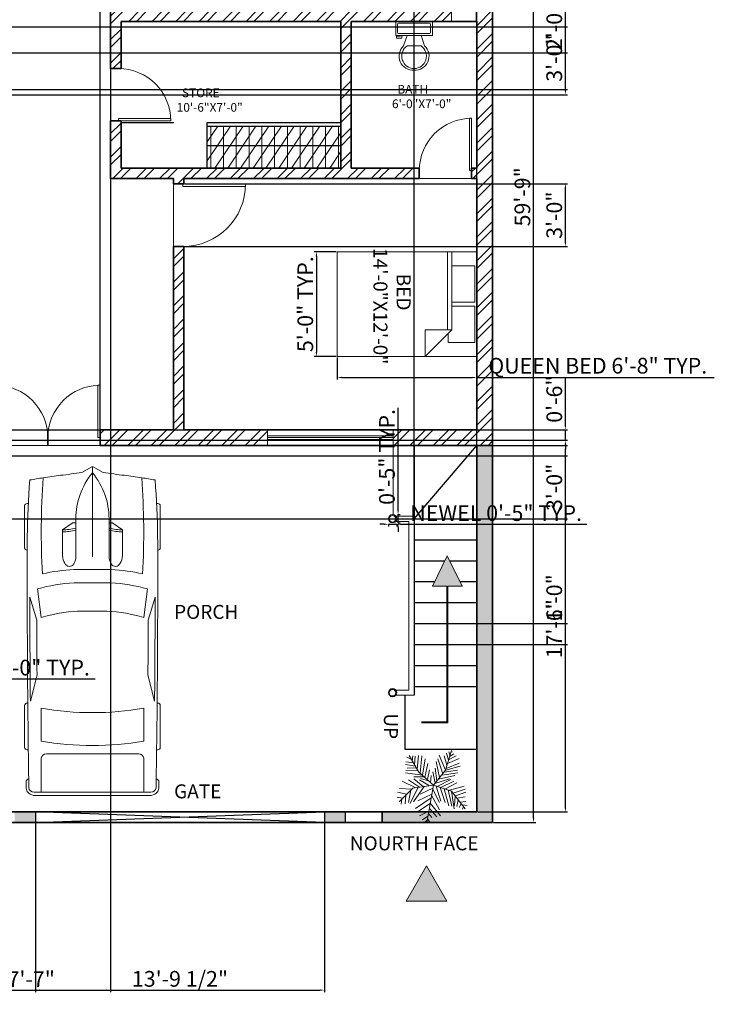
# Model space of a CAD drawing. Units: inches. Extents: x 177 to 1423, y 532 to 2503.
# Tile 3 of 5: x 453 to 852, y 532 to 1096. Entities that reach past the tile are written whole.
import ezdxf

# ---------------------------------------------------------------- set-up
doc = ezdxf.new("R2010")
doc.units = ezdxf.units.IN
for name, color, linetype, lineweight in [('A-ANNO-DIMS', 2, 'Continuous', 18), ('A-ANNO-SYMB', 7, 'Continuous', 18), ('A-ANNO-TEXT', 7, 'Continuous', 18), ('A-AREA-IDEN', 7, 'Continuous', 18), ('A-DOOR', 4, 'Continuous', 18), ('A-FLOR-CASE', 8, 'Continuous', 25), ('A-FLOR-CASE-PATT', 252, 'Continuous', 13), ('A-FLOR-FIXT', 9, 'Continuous', 18), ('A-FLOR-RAIL', 8, 'Continuous', 18), ('A-FLOR-STRS', 7, 'Continuous', 25), ('A-FURN', 8, 'Continuous', 18), ('A-GLAZ', 244, 'Continuous', 18), ('A-SITE-GATE', 244, 'Continuous', 25), ('A-WALL', 7, 'Continuous', 35), ('A-WALL-PATT', 252, 'Continuous', 13), ('C-SITE-VEHI', 9, 'Continuous', 13), ('L-PLNT', 94, 'Continuous', 13)]:
    doc.layers.add(name, color=color, linetype=linetype, lineweight=lineweight)
doc.styles.get("Standard").update_dxf_attribs({"font": 'arial.ttf'})
doc.dimstyles.new('ISO-25', dxfattribs={"dimtxt": 9, "dimasz": 2.5, "dimexe": 1.25, "dimexo": 0.625, "dimtad": 1, "dimlunit": 3, "dimtxsty": 'Standard', "dimcen": 2.5, "dimadec": 0, "dimazin": 0, "dimtfac": 1, "dimtmove": 0, "dimatfit": 3, "dimfxl": 1, "dimarcsym": 0})

# ---------------------------------------------------------------- blocks, each defined once
blk = doc.blocks.new('*U2')
for p, q in [((0, 0), (0, -6)), ((40, 0), (40, -6))]:
    blk.add_line(p, q)
blk.add_lwpolyline([(0, 0), (0, 40), (1.75, 40), (1.75, 0)], close=True)
blk.add_arc((0, 0), 40, 0, 90)
blk = doc.blocks.new('*U5')
for p, q in [((0, 0), (0, -6)), ((-40, 0), (-40, -6))]:
    blk.add_line(p, q)
blk.add_lwpolyline([(0, 0), (0, 40), (-1.75, 40), (-1.75, 0)], close=True)
blk.add_arc((0, 0), 40, 90, 180)
blk = doc.blocks.new('Bed - Queen')
for p, q in [((0, -80.00003), (0, 0)), ((0, 0), (59.99999, 0)), ((59.99999, 0), (59.99999, -80.00003)), ((7.99999, -1.2), (28.79998, -1.2)), ((7.99999, -14.4), (7.99999, -1.2)), ((28.79998, -1.2), (28.79998, -14.4)), ((31.19999, -1.2), (51.99999, -1.2)), ((31.19999, -14.4), (31.19999, -1.2)), ((51.99999, -1.2), (51.99999, -16.4)), ((0, -14.4), (44.8, -14.4)), ((44.8, -16.8), (0, -16.8)), ((59.99999, -29.6), (44.8, -14.4)), ((44.8, -14.4), (44.8, -29.6)), ((51.99999, -16.4), (46.79936, -16.4)), ((44.8, -29.6), (59.99999, -29.6)), ((59.99999, -80.00003), (0, -80.00003))]:
    blk.add_line(p, q)
blk = doc.blocks.new('*U9')
for p, q in [((9.5, -6), (9.5, -2)), ((-10, -8.5), (-8, -8.5)), ((-10, -9.5), (-10, -8.5)), ((-7, -9.5), (-10, -9.5)), ((-8, -8.5), (-8, -8)), ((-7, -8), (-7, -9.5)), ((-4, -8), (-6, -14)), ((4, -8), (6, -14)), ((4, -14), (-4, -14))]:
    blk.add_line(p, q)
blk.add_lwpolyline([(10.5, -8), (10.5, 0), (-10.5, 0), (-10.5, -8)], close=True)
for points in [[(-9.5, -2), (-9.5, -6)], [(8.5, -1), (-8.5, -1)], [(-8.5, -7), (8.5, -7)]]:
    blk.add_lwpolyline(points)
for centre, radius, start, end in [((-8.625, -1.875), 0.8839, 81.8699, 188.1301), ((8.625, -1.875), 0.8839, 351.8699, 98.1301), ((-8.625, -6.125), 0.8839, 171.869898, 278.1301), ((8.625, -6.125), 0.8839, 261.8699, 8.1301), ((-0.4772, -19.9188), 8.0953, 133.01722, 273.38), ((0.0374, -19.8731), 7.127, 124.50543, 269.7), ((-0.0373, -19.8731), 7.127, 270.3, 55.4946), ((0.4773, -19.9188), 8.0953, 266.62, 46.9828)]:
    blk.add_arc(centre, radius, start, end)
blk = doc.blocks.new('*U14')
for p, q in [((21.1, 37.41), (21.1, 36.83)), ((46.55, 38.89), (22.35, 38.89)), ((47.8, 37.39), (47.8, 37.41)), ((87.99, 31.87), (74.76, 35.92)), ((134.31, 35.6), (119.29, 31.78)), ((135.45, 37.07), (135.45, 37.41)), ((136.7, 38.89), (160.9, 38.89)), ((162.15, 37.41), (162.15, 36.77)), ((70.03, 31.54), (86.41, 29.35)), ((138.42, 29.35), (157.25, 29.35)), ((186.47, 29.35), (167.01, 29.35)), ((186.47, -33.5), (186.47, 33.5)), ((188.4, -32.76), (188.4, 32.76)), ((164.52, 26.39), (164.52, -26.39)), ((32.27, 11.63), (36.13, 17.17)), ((36.13, 17.17), (50.94, 17.17)), ((3.27, 6.13), (0.1, 0.41)), ((29.77, 9.51), (51.68, 9.51)), ((32.12, 9.51), (32.12, 11.15)), ((58.92, -10.77), (58.92, 10.77)), ((66.55, -10.53), (66.55, 10.53)), ((82.74, 8.5), (82.74, -8.5)), ((186.47, -10.53), (186.47, 10.53)), ((0, 0), (51.68, 0)), ((0.1, -0.41), (3.27, -6.13)), ((29.77, -9.51), (51.68, -9.51)), ((32.12, -9.51), (32.12, -11.15)), ((32.27, -11.63), (36.13, -17.17)), ((36.13, -17.17), (50.94, -17.17)), ((86.41, -29.35), (70.03, -31.54)), ((87.99, -31.87), (74.76, -35.92)), ((134.31, -35.6), (119.29, -31.78)), ((157.25, -29.35), (138.42, -29.35)), ((167.01, -29.35), (186.47, -29.35)), ((21.1, -37.41), (21.1, -36.83)), ((46.55, -38.89), (22.35, -38.89)), ((47.8, -37.39), (47.8, -37.41)), ((135.45, -37.07), (135.45, -37.41)), ((136.7, -38.89), (160.9, -38.89)), ((162.15, -37.41), (162.15, -36.77))]:
    blk.add_line(p, q)
for centre, major_axis, ratio, start_param, end_param in [((266.03, -27.52), (0, 313.31), 0.842304, 1.367076, 1.39176), ((41.19, -490.86), (0, 528.23), 0.842304, 0.00281, 0.075598), ((22.35, 37.41), (0, -1.48), 0.842304, 3.141593, 4.712389), ((64.48, -10555.62), (0, 10593.03), 0.842304, -0.013397, 0.002797), ((46.55, 37.41), (0, 1.48), 0.842304, -1.570796, 0), ((64.48, -10555.62), (0, -10591.55), 0.842304, 3.133765, 3.140441), ((136.7, 37.41), (0, -1.48), 0.842304, 3.141593, 4.712389), ((160.9, 37.41), (0, 1.48), 0.842304, -1.570796, 0), ((180.63, 35.84), (0, 2.22), 0.842304, -0.013017, 1.249894), ((64.48, -10556.36), (0, 10595.31), 0.842304, -0.013397, -0.013017), ((183.98, 33.5), (0, -2.96), 0.842304, 1.570796, 3.128196), ((183.98, 32.76), (0, -5.25), 0.842304, 1.570796, 3.128196), ((259.18, -27.52), (0, -305.3), 0.842304, 4.528606, 4.561838), ((37.47, -593.96), (0, -623.33), 0.842304, 3.096046, 3.200911), ((134.4, 5.39), (0, -89.78), 0.842304, 4.449482, 4.652344), ((135.29, 5.39), (0, 81.77), 0.842304, 1.245306, 1.50788), ((149.6, 2.8), (0, -79.58), 0.842304, 4.372215, 4.640744), ((95.79, -3666.35), (0, -3698.24), 0.842304, 3.134049, 3.144098), ((17.08, 0), (0, 147.02), 0.842304, 4.511394, 4.913384), ((35.91, 0), (0, 147.02), 0.842304, 4.511394, 4.913384), ((167.01, 26.39), (0, 2.96), 0.842304, 0, 1.570796), ((-204.49, 52.4), (0, -250.96), 0.842304, 1.385369, 1.434372), ((13.04, 17.01), (0, 27.42), 0.842304, 4.435146, 4.718221), ((14.2, 17.01), (0, 27.42), 0.842304, 4.435146, 4.718221), ((50.79, 13.34), (6.34, -0.36), 0.603834, -1.395552, 1.581315), ((32.75, 11.15), (0, 0.74), 0.842304, 0.879714, 1.570796), ((29.77, -46.66), (0, 56.17), 0.842304, 0, 0.590319), ((0.62, 0), (0, -0.74), 0.842304, 4.131459, 5.293319), ((29.77, 46.66), (0, 56.17), 0.842304, 2.551274, 3.141593), ((-204.49, -52.4), (0, 250.96), 0.842304, -1.434372, -1.385369), ((32.75, -11.15), (0, -0.74), 0.842304, 4.712389, 5.403472), ((13.04, -17.01), (0, -27.42), 0.842304, 1.564964, 1.848039), ((14.2, -17.01), (0, -27.42), 0.842304, 1.564964, 1.848039), ((134.4, -5.39), (0, -89.78), 0.842304, -1.510751, -1.307889), ((135.29, -5.39), (0, -81.77), 0.842304, -1.50788, -1.245306), ((149.6, -2.8), (0, -79.58), 0.842304, -1.499151, -1.230623), ((259.18, 27.52), (0, 305.3), 0.842304, 1.721348, 1.754579), ((167.01, -26.39), (0, -2.96), 0.842304, 4.712389, 6.283185), ((266.03, 27.52), (0, 313.31), 0.842304, 1.749832, 1.774517), ((37.47, 593.96), (0, -623.33), 0.842304, -0.059319, 0.045547), ((95.79, 3666.35), (0, -3698.24), 0.842304, -0.002505, 0.007544), ((183.98, -33.5), (0, 2.96), 0.842304, 3.15499, 4.712389), ((183.98, -32.76), (0, -5.25), 0.842304, 0.013397, 1.570796), ((41.19, 490.86), (0, -528.23), 0.842304, -0.075598, -0.00281), ((22.35, -37.41), (0, 1.48), 0.842304, 1.570796, 3.141593), ((64.48, 10555.62), (0, 10593.03), 0.842304, 3.138796, 3.15499), ((46.55, -37.41), (0, -1.48), 0.842304, 0, 1.570796), ((64.48, 10555.62), (0, -10591.55), 0.842304, 0.001152, 0.007828), ((136.7, -37.41), (0, -1.48), 0.842304, -1.570796, 0), ((160.9, -37.41), (0, 1.48), 0.842304, 3.141593, 4.712389), ((180.63, -35.84), (0, -2.22), 0.842304, -1.249894, 0.013017), ((64.48, 10556.36), (0, 10595.31), 0.842304, 3.15461, 3.15499)]:
    blk.add_ellipse(centre, major_axis=major_axis, ratio=ratio, start_param=start_param, end_param=end_param)
at = {"extrusion": (0, 0, -1)}
blk.add_ellipse((50.79, -13.34), major_axis=(6.34, 0.36), ratio=0.603834, start_param=-1.395552, end_param=1.581315, dxfattribs=at)
blk = doc.blocks.new('*D16')
at = {"layer": 'A-ANNO-DIMS', "color": 0, "lineweight": -2, "transparency": 16777216}
for p, q in [((725.18, 1353.15), (749.29, 1353.15)), ((748.04, 638.65), (748.04, 1350.65)), ((725.18, 636.15), (749.29, 636.15))]:
    blk.add_line(p, q, dxfattribs=at)
at = {"layer": 'A-ANNO-DIMS', "color": 0, "transparency": 16777216}
for points in [[(747.63, 1350.65), (748.46, 1350.65), (748.04, 1353.15)], [(747.63, 638.65), (748.46, 638.65), (748.04, 636.15)]]:
    blk.add_solid(points, dxfattribs=at)
at = {"layer": 'Defpoints', "color": 0, "transparency": 16777216}
for p in [(724.55, 1353.15), (748.04, 1353.15), (724.55, 636.15)]:
    blk.add_point(p, dxfattribs=at)
at = {"layer": 'A-ANNO-DIMS', "color": 0, "transparency": 16777216, "insert": (742.82, 994.65), "char_height": 9, "attachment_point": 5, "rotation": 90}
blk.add_mtext('59\'-9"', dxfattribs=at)
blk = doc.blocks.new('*U11')
for p, q in [((-7.288, 39.707), (-21.778, 46.673)), ((-8.737, 47.138), (-17.069, 52.711)), ((-10.186, 53.64), (-13.084, 55.962)), ((0, 0), (-10.5, 57)), ((-9.099, 51.782), (-6.563, 55.962)), ((-7.65, 43.423), (-2.578, 49.46)), ((-5.839, 35.992), (4.667, 48.067)), ((-5.114, 27.632), (10.463, 46.673)), ((-3.665, 19.273), (-27.574, 35.527)), ((-5.114, 28.097), (-24.676, 40.636)), ((-2.941, 16.486), (8.652, 37.85)), ((16.259, 5.805), (23.142, 31.348)), ((22.055, 7.198), (27.489, 32.277)), ((27, 9), (48, 36)), ((27.127, 9.056), (31.112, 35.992)), ((31.836, 30.883), (32.561, 16.486)), ((35.096, 32.741), (37.27, 22.524)), ((38.719, 34.134), (41.979, 28.561)), ((43.791, 29.954), (51.036, 30.883)), ((44.153, 36.456), (45.239, 32.741)), ((-47.498, 19.737), (-55.83, 18.344)), ((-31.5, 4.5), (-52.5, 25.5)), ((-48.585, 21.131), (-49.309, 29.026)), ((-43.513, 28.561), (-42.427, 15.558)), ((-38.442, 26.239), (-34.819, 7.663)), ((-35.544, 28.097), (-24.314, 3.947)), ((-14.533, 2.09), (-30.834, 25.31)), ((-24.314, 23.917), (-2.941, 13.7)), ((-1.129, 6.734), (9.014, 26.704)), ((3.942, 1.625), (11.187, 24.381)), ((10.101, 3.483), (17.708, 26.239)), ((33.285, 16.486), (48.862, 10.913)), ((36.183, 19.737), (48.137, 17.88)), ((40.53, 25.775), (48.862, 24.846)), ((-40.615, 13.7), (-55.105, 10.913)), ((-33.37, 6.269), (-52.207, 5.34)), ((-28.299, 3.483), (-47.86, -5.805)), ((-21.416, 3.018), (-38.079, -8.128)), ((0, 0), (-31.5, 4.5)), ((-15.982, 2.09), (-30.11, -9.521)), ((0, 0), (-22.5, -19.5)), ((-6.563, 1.161), (-21.416, -8.128)), ((-20.691, 13.7), (-1.129, 4.876)), ((0, 0), (27, 9)), ((0, 0), (18, -22.5)), ((6.478, 1.625), (26.04, -8.592)), ((11.187, 3.483), (30.749, -5.805)), ((18.07, 5.805), (35.096, -3.483)), ((24.229, 7.663), (46.688, 1.625)), ((29.662, 12.307), (48.137, 6.269)), ((-15.257, -12.772), (-30.11, -12.772)), ((-6.563, -5.805), (-19.967, -9.985)), ((-13.446, -11.378), (-8.737, -32.741)), ((-9.461, -8.592), (-6.201, -23.453)), ((-4.752, -3.483), (-3.665, -14.629)), ((2.493, -3.019), (-1.491, -20.202)), ((1.769, -2.555), (24.229, -9.521)), ((5.029, -6.27), (2.131, -25.775)), ((9.014, -11.378), (3.58, -35.992)), ((7.565, -9.056), (32.198, -14.629)), ((-17.431, -15.094), (-42.789, -18.809)), ((-28.299, -29.026), (-42.789, -31.348)), ((-24.314, -21.596), (-42.427, -22.06)), ((-26.849, -26.24), (-40.253, -25.775)), ((-22.5, -19.5), (-37.5, -45)), ((-25.038, -23.918), (-22.865, -45.281)), ((-20.691, -18.345), (-17.793, -44.352)), ((-17.069, -15.094), (-12.721, -40.172)), ((14.085, -16.951), (6.478, -40.172)), ((18.07, -22.524), (8.289, -45.745)), ((12.274, -15.094), (36.907, -18.809)), ((16.259, -19.738), (36.183, -22.989)), ((18, -22.5), (27, -52.5)), ((18.433, -22.524), (40.53, -29.026)), ((19.157, -25.311), (38.719, -33.206)), ((-30.834, -34.135), (-42.427, -35.528)), ((-34.457, -39.708), (-40.978, -42.494)), ((-32.646, -36.921), (-31.921, -44.352)), ((-29.023, -30.884), (-27.936, -43.887)), ((20.244, -30.419), (15.897, -44.816)), ((22.78, -37.85), (19.519, -48.532)), ((21.331, -32.741), (39.081, -40.636)), ((22.78, -38.314), (34.372, -44.816)), ((24.591, -43.423), (30.749, -47.603)), ((24.591, -45.745), (23.142, -50.854)), ((26.764, -49.925), (28.213, -50.854))]:
    blk.add_line(p, q)
blk = doc.blocks.new('WIN-GLAZING-72IN')
for p, q in [((72, 2), (0, 2)), ((72, 1), (0, 1)), ((72, 0), (0, 0))]:
    blk.add_line(p, q)
blk = doc.blocks.new('STAIR-NEWEL-ROUND')
for radius in [2.39, 1.89]:
    blk.add_circle((2.39, 2.39), radius)
blk = doc.blocks.new('*D22')
at = {"layer": 'A-ANNO-DIMS', "color": 0, "lineweight": -2, "transparency": 16777216}
for p, q in [((635.55, 902.53), (635.55, 889.9)), ((715.55, 902.53), (715.55, 889.9)), ((638.05, 891.15), (713.05, 891.15)), ((715.55, 891.15), (851.69, 891.15))]:
    blk.add_line(p, q, dxfattribs=at)
at = {"layer": 'A-ANNO-DIMS', "color": 0, "transparency": 16777216}
for points in [[(638.05, 891.57), (638.05, 890.74), (635.55, 891.15)], [(713.05, 891.57), (713.05, 890.74), (715.55, 891.15)]]:
    blk.add_solid(points, dxfattribs=at)
at = {"layer": 'Defpoints', "color": 0, "transparency": 16777216}
for p in [(635.55, 903.15), (715.55, 903.15), (715.55, 891.15)]:
    blk.add_point(p, dxfattribs=at)
at = {"layer": 'A-ANNO-DIMS', "color": 0, "transparency": 16777216, "insert": (784.87, 896.71), "char_height": 9, "attachment_point": 5}
blk.add_mtext('QUEEN BED 6\'-8" TYP.', dxfattribs=at)
blk = doc.blocks.new('*D23')
at = {"layer": 'A-ANNO-DIMS', "color": 0, "lineweight": -2, "transparency": 16777216}
for p, q in [((634.93, 963.15), (622.3, 963.15)), ((623.55, 960.65), (623.55, 905.65)), ((634.93, 903.15), (622.3, 903.15))]:
    blk.add_line(p, q, dxfattribs=at)
at = {"layer": 'A-ANNO-DIMS', "color": 0, "transparency": 16777216}
for points in [[(623.13, 960.65), (623.97, 960.65), (623.55, 963.15)], [(623.13, 905.65), (623.97, 905.65), (623.55, 903.15)]]:
    blk.add_solid(points, dxfattribs=at)
at = {"layer": 'Defpoints', "color": 0, "transparency": 16777216}
for p in [(635.55, 963.15), (623.55, 903.15), (635.55, 903.15)]:
    blk.add_point(p, dxfattribs=at)
at = {"layer": 'A-ANNO-DIMS', "color": 0, "transparency": 16777216, "insert": (618.33, 933.15), "char_height": 9, "attachment_point": 5, "rotation": 90}
blk.add_mtext('5\'-0" TYP.', dxfattribs=at)
blk = doc.blocks.new('*D24')
at = {"layer": 'A-ANNO-DIMS', "color": 0, "lineweight": -2, "transparency": 16777216}
for p, q in [((307.55, 708.28), (307.55, 719.7)), ((310.05, 718.45), (377.05, 718.45)), ((379.55, 708.28), (379.55, 719.7)), ((379.55, 718.45), (496.7, 718.45))]:
    blk.add_line(p, q, dxfattribs=at)
at = {"layer": 'A-ANNO-DIMS', "color": 0, "transparency": 16777216}
for points in [[(310.05, 718.87), (310.05, 718.04), (307.55, 718.45)], [(377.05, 718.87), (377.05, 718.04), (379.55, 718.45)]]:
    blk.add_solid(points, dxfattribs=at)
at = {"layer": 'Defpoints', "color": 0, "transparency": 16777216}
for p in [(379.55, 718.45), (307.55, 707.65), (379.55, 707.65)]:
    blk.add_point(p, dxfattribs=at)
at = {"layer": 'A-ANNO-DIMS', "color": 0, "transparency": 16777216, "insert": (439.37, 723.73), "char_height": 9, "attachment_point": 5}
blk.add_mtext('GLAZING 6\'-0" TYP.', dxfattribs=at)
blk = doc.blocks.new('*D28')
at = {"layer": 'A-ANNO-DIMS', "color": 0, "lineweight": -2, "transparency": 16777216}
for p, q in [((662.36, 807.04), (659.86, 807.04)), ((664.86, 807.13), (664.86, 805.79)), ((664.86, 807.04), (669.65, 807.04)), ((669.65, 807.13), (669.65, 805.79)), ((672.15, 807.04), (778.53, 807.04))]:
    blk.add_line(p, q, dxfattribs=at)
at = {"layer": 'A-ANNO-DIMS', "color": 0, "transparency": 16777216}
for points in [[(662.36, 807.46), (662.36, 806.62), (664.86, 807.04)], [(672.15, 807.46), (672.15, 806.62), (669.65, 807.04)]]:
    blk.add_solid(points, dxfattribs=at)
at = {"layer": 'Defpoints', "color": 0, "transparency": 16777216}
for p in [(664.86, 807.76), (669.65, 807.76), (669.65, 807.04)]:
    blk.add_point(p, dxfattribs=at)
at = {"layer": 'A-ANNO-DIMS', "color": 0, "transparency": 16777216, "insert": (726.59, 812.26), "char_height": 9, "attachment_point": 5}
blk.add_mtext('NEWEL 0\'-5" TYP.', dxfattribs=at)
blk = doc.blocks.new('*D29')
at = {"layer": 'A-ANNO-DIMS', "color": 0, "lineweight": -2, "transparency": 16777216}
for p, q in [((670.37, 815.05), (670.37, 873.66)), ((670.28, 812.55), (671.62, 812.55)), ((670.37, 807.76), (670.37, 812.55)), ((670.28, 807.76), (671.62, 807.76)), ((670.37, 805.26), (670.37, 802.76))]:
    blk.add_line(p, q, dxfattribs=at)
at = {"layer": 'A-ANNO-DIMS', "color": 0, "transparency": 16777216}
for points in [[(669.95, 815.05), (670.79, 815.05), (670.37, 812.55)], [(669.95, 805.26), (670.79, 805.26), (670.37, 807.76)]]:
    blk.add_solid(points, dxfattribs=at)
at = {"layer": 'Defpoints', "color": 0, "transparency": 16777216}
for p in [(669.65, 812.55), (670.37, 812.55), (669.65, 807.76)]:
    blk.add_point(p, dxfattribs=at)
at = {"layer": 'A-ANNO-DIMS', "color": 0, "transparency": 16777216, "insert": (665.15, 845.6), "char_height": 9, "attachment_point": 5, "rotation": 90}
blk.add_mtext('0\'-5" TYP.', dxfattribs=at)
blk = doc.blocks.new('*D35')
at = {"layer": 'A-ANNO-DIMS', "color": 0, "lineweight": -2, "transparency": 16777216}
for p, q in [((462.59, 635.53), (462.59, 538.84)), ((628.1, 635.53), (628.1, 538.84)), ((465.09, 540.09), (625.6, 540.09))]:
    blk.add_line(p, q, dxfattribs=at)
at = {"layer": 'A-ANNO-DIMS', "color": 0, "transparency": 16777216}
for points in [[(465.09, 540.51), (465.09, 539.68), (462.59, 540.09)], [(625.6, 540.51), (625.6, 539.68), (628.1, 540.09)]]:
    blk.add_solid(points, dxfattribs=at)
at = {"layer": 'Defpoints', "color": 0, "transparency": 16777216}
for p in [(462.59, 636.15), (628.1, 636.15), (628.1, 540.09)]:
    blk.add_point(p, dxfattribs=at)
at = {"layer": 'A-ANNO-DIMS', "color": 0, "transparency": 16777216, "insert": (545.34, 545.37), "char_height": 9, "attachment_point": 5}
blk.add_mtext('13\'-9 1/2"', dxfattribs=at)
blk = doc.blocks.new('*D36')
at = {"layer": 'A-ANNO-DIMS', "color": 0, "lineweight": -2, "transparency": 16777216}
for p, q in [((766.3, 750.15), (766.3, 776.98)), ((716.18, 750.15), (767.55, 750.15)), ((766.3, 740.65), (766.3, 747.65)), ((716.18, 738.15), (767.55, 738.15))]:
    blk.add_line(p, q, dxfattribs=at)
at = {"layer": 'A-ANNO-DIMS', "color": 0, "transparency": 16777216}
for points in [[(765.88, 747.65), (766.72, 747.65), (766.3, 750.15)], [(765.88, 740.65), (766.72, 740.65), (766.3, 738.15)]]:
    blk.add_solid(points, dxfattribs=at)
at = {"layer": 'Defpoints', "color": 0, "transparency": 16777216}
for p in [(715.55, 750.15), (766.3, 750.15), (715.55, 738.15)]:
    blk.add_point(p, dxfattribs=at)
at = {"layer": 'A-ANNO-DIMS', "color": 0, "transparency": 16777216, "insert": (761.08, 764.82), "char_height": 9, "attachment_point": 5, "rotation": 90}
blk.add_mtext('1\'-0"', dxfattribs=at)
blk = doc.blocks.new('*D37')
at = {"layer": 'A-ANNO-DIMS', "color": 0, "lineweight": -2, "transparency": 16777216}
for p, q in [((716.18, 852.15), (767.55, 852.15)), ((766.3, 644.65), (766.3, 849.65)), ((716.18, 642.15), (767.55, 642.15))]:
    blk.add_line(p, q, dxfattribs=at)
at = {"layer": 'A-ANNO-DIMS', "color": 0, "transparency": 16777216}
for points in [[(765.88, 849.65), (766.72, 849.65), (766.3, 852.15)], [(765.88, 644.65), (766.72, 644.65), (766.3, 642.15)]]:
    blk.add_solid(points, dxfattribs=at)
at = {"layer": 'Defpoints', "color": 0, "transparency": 16777216}
for p in [(715.55, 852.15), (766.3, 852.15), (715.55, 642.15)]:
    blk.add_point(p, dxfattribs=at)
at = {"layer": 'A-ANNO-DIMS', "color": 0, "transparency": 16777216, "insert": (761.08, 747.15), "char_height": 9, "attachment_point": 5, "rotation": 90}
blk.add_mtext('17\'-6"', dxfattribs=at)
blk = doc.blocks.new('*D38')
at = {"layer": 'A-ANNO-DIMS', "color": 0, "lineweight": -2, "transparency": 16777216}
for p, q in [((679.55, 810.78), (679.55, 1447.15)), ((682.05, 1445.9), (713.05, 1445.9)), ((715.55, 810.78), (715.55, 1447.15))]:
    blk.add_line(p, q, dxfattribs=at)
at = {"layer": 'A-ANNO-DIMS', "color": 0, "transparency": 16777216}
for points in [[(682.05, 1446.32), (682.05, 1445.49), (679.55, 1445.9)], [(713.05, 1446.32), (713.05, 1445.49), (715.55, 1445.9)]]:
    blk.add_solid(points, dxfattribs=at)
at = {"layer": 'Defpoints', "color": 0, "transparency": 16777216}
for p in [(715.55, 1445.9), (679.55, 810.15), (715.55, 810.15)]:
    blk.add_point(p, dxfattribs=at)
at = {"layer": 'A-ANNO-DIMS', "color": 0, "transparency": 16777216, "insert": (697.55, 1451.13), "char_height": 9, "attachment_point": 5}
blk.add_mtext('3\'-0"', dxfattribs=at)
blk = doc.blocks.new('*D40')
at = {"layer": 'A-ANNO-DIMS', "color": 0, "lineweight": -2, "transparency": 16777216}
for p, q in [((414.55, 1172.53), (414.55, 538.84)), ((505.55, 1172.53), (505.55, 538.84)), ((417.05, 540.09), (503.05, 540.09))]:
    blk.add_line(p, q, dxfattribs=at)
at = {"layer": 'A-ANNO-DIMS', "color": 0, "transparency": 16777216}
for points in [[(417.05, 540.51), (417.05, 539.68), (414.55, 540.09)], [(503.05, 540.51), (503.05, 539.68), (505.55, 540.09)]]:
    blk.add_solid(points, dxfattribs=at)
at = {"layer": 'Defpoints', "color": 0, "transparency": 16777216}
for p in [(414.55, 1173.15), (505.55, 1173.15), (505.55, 540.09)]:
    blk.add_point(p, dxfattribs=at)
at = {"layer": 'A-ANNO-DIMS', "color": 0, "transparency": 16777216, "insert": (460.05, 545.22), "char_height": 9, "attachment_point": 5}
blk.add_mtext('7\'-7"', dxfattribs=at)
blk = doc.blocks.new('*D41')
at = {"layer": 'A-ANNO-DIMS', "color": 0, "lineweight": -2, "transparency": 16777216}
for p, q in [((439.55, 861.78), (439.55, 1447.15)), ((442.05, 1445.9), (497.05, 1445.9)), ((499.55, 861.78), (499.55, 1447.15))]:
    blk.add_line(p, q, dxfattribs=at)
at = {"layer": 'A-ANNO-DIMS', "color": 0, "transparency": 16777216}
for points in [[(442.05, 1446.32), (442.05, 1445.49), (439.55, 1445.9)], [(497.05, 1446.32), (497.05, 1445.49), (499.55, 1445.9)]]:
    blk.add_solid(points, dxfattribs=at)
at = {"layer": 'Defpoints', "color": 0, "transparency": 16777216}
for p in [(499.55, 1445.9), (439.55, 861.15), (499.55, 861.15)]:
    blk.add_point(p, dxfattribs=at)
at = {"layer": 'A-ANNO-DIMS', "color": 0, "transparency": 16777216, "insert": (469.55, 1451.12), "char_height": 9, "attachment_point": 5}
blk.add_mtext('5\'-0"', dxfattribs=at)
blk = doc.blocks.new('*D43')
at = {"layer": 'A-ANNO-DIMS', "color": 0, "lineweight": -2, "transparency": 16777216}
for p, q in [((766.3, 863.65), (766.3, 891.33)), ((299.18, 861.15), (767.55, 861.15)), ((766.3, 855.15), (766.3, 861.15)), ((299.18, 855.15), (767.55, 855.15)), ((766.3, 852.65), (766.3, 850.15))]:
    blk.add_line(p, q, dxfattribs=at)
at = {"layer": 'A-ANNO-DIMS', "color": 0, "transparency": 16777216}
for points in [[(765.88, 863.65), (766.72, 863.65), (766.3, 861.15)], [(765.88, 852.65), (766.72, 852.65), (766.3, 855.15)]]:
    blk.add_solid(points, dxfattribs=at)
at = {"layer": 'Defpoints', "color": 0, "transparency": 16777216}
for p in [(298.55, 861.15), (766.3, 861.15), (298.55, 855.15)]:
    blk.add_point(p, dxfattribs=at)
at = {"layer": 'A-ANNO-DIMS', "color": 0, "transparency": 16777216, "insert": (761.08, 878.74), "char_height": 9, "attachment_point": 5, "rotation": 90}
blk.add_mtext('0\'-6"', dxfattribs=at)
blk = doc.blocks.new('*D44')
at = {"layer": 'A-ANNO-DIMS', "color": 0, "lineweight": -2, "transparency": 16777216}
for p, q in [((437.18, 846.15), (767.55, 846.15)), ((766.3, 812.65), (766.3, 843.65)), ((437.18, 810.15), (767.55, 810.15))]:
    blk.add_line(p, q, dxfattribs=at)
at = {"layer": 'A-ANNO-DIMS', "color": 0, "transparency": 16777216}
for points in [[(765.88, 843.65), (766.72, 843.65), (766.3, 846.15)], [(765.88, 812.65), (766.72, 812.65), (766.3, 810.15)]]:
    blk.add_solid(points, dxfattribs=at)
at = {"layer": 'Defpoints', "color": 0, "transparency": 16777216}
for p in [(436.55, 846.15), (766.3, 846.15), (436.55, 810.15)]:
    blk.add_point(p, dxfattribs=at)
at = {"layer": 'A-ANNO-DIMS', "color": 0, "transparency": 16777216, "insert": (761.08, 828.15), "char_height": 9, "attachment_point": 5, "rotation": 90}
blk.add_mtext('3\'-0"', dxfattribs=at)
blk = doc.blocks.new('*D48')
at = {"layer": 'A-ANNO-DIMS', "color": 0, "lineweight": -2, "transparency": 16777216}
for p, q in [((766.3, 1077.15), (766.3, 1104.98)), ((338.12, 1077.15), (767.55, 1077.15)), ((766.3, 1055.65), (766.3, 1074.65)), ((338.12, 1053.15), (767.55, 1053.15))]:
    blk.add_line(p, q, dxfattribs=at)
at = {"layer": 'A-ANNO-DIMS', "color": 0, "transparency": 16777216}
for points in [[(765.88, 1074.65), (766.72, 1074.65), (766.3, 1077.15)], [(765.88, 1055.65), (766.72, 1055.65), (766.3, 1053.15)]]:
    blk.add_solid(points, dxfattribs=at)
at = {"layer": 'Defpoints', "color": 0, "transparency": 16777216}
for p in [(337.49, 1077.15), (766.3, 1077.15), (337.49, 1053.15)]:
    blk.add_point(p, dxfattribs=at)
at = {"layer": 'A-ANNO-DIMS', "color": 0, "transparency": 16777216, "insert": (761.08, 1092.32), "char_height": 9, "attachment_point": 5, "rotation": 90}
blk.add_mtext('2\'-0"', dxfattribs=at)
blk = doc.blocks.new('*D52')
at = {"layer": 'A-ANNO-DIMS', "color": 0, "lineweight": -2, "transparency": 16777216}
for p, q in [((409.18, 1092.15), (767.55, 1092.15)), ((766.3, 1058.65), (766.3, 1089.65)), ((409.18, 1056.15), (767.55, 1056.15))]:
    blk.add_line(p, q, dxfattribs=at)
at = {"layer": 'A-ANNO-DIMS', "color": 0, "transparency": 16777216}
for points in [[(765.88, 1089.65), (766.72, 1089.65), (766.3, 1092.15)], [(765.88, 1058.65), (766.72, 1058.65), (766.3, 1056.15)]]:
    blk.add_solid(points, dxfattribs=at)
at = {"layer": 'Defpoints', "color": 0, "transparency": 16777216}
for p in [(408.55, 1092.15), (766.3, 1092.15), (408.55, 1056.15)]:
    blk.add_point(p, dxfattribs=at)
at = {"layer": 'A-ANNO-DIMS', "color": 0, "transparency": 16777216, "insert": (761.08, 1074.15), "char_height": 9, "attachment_point": 5, "rotation": 90}
blk.add_mtext('3\'-0"', dxfattribs=at)
blk = doc.blocks.new('*D57')
at = {"layer": 'A-ANNO-DIMS', "color": 0, "lineweight": -2, "transparency": 16777216}
for p, q in [((548.18, 1002.15), (767.55, 1002.15)), ((766.3, 968.65), (766.3, 999.65)), ((548.18, 966.15), (767.55, 966.15))]:
    blk.add_line(p, q, dxfattribs=at)
at = {"layer": 'A-ANNO-DIMS', "color": 0, "transparency": 16777216}
for points in [[(765.88, 999.65), (766.72, 999.65), (766.3, 1002.15)], [(765.88, 968.65), (766.72, 968.65), (766.3, 966.15)]]:
    blk.add_solid(points, dxfattribs=at)
at = {"layer": 'Defpoints', "color": 0, "transparency": 16777216}
for p in [(547.55, 1002.15), (766.3, 1002.15), (547.55, 966.15)]:
    blk.add_point(p, dxfattribs=at)
at = {"layer": 'A-ANNO-DIMS', "color": 0, "transparency": 16777216, "insert": (761.08, 984.15), "char_height": 9, "attachment_point": 5, "rotation": 90}
blk.add_mtext('3\'-0"', dxfattribs=at)

msp = doc.modelspace()

# ---------------------------------------------------------------- hatches: boundary and pattern name
at = {"layer": 'A-ANNO-SYMB'}
h = msp.add_hatch(color=256, dxfattribs=at)
h.dxf.hatch_style = 1
h.paths.add_polyline_path([(698.607, 788.878), (690.096, 771.466), (698.307, 771.466), (698.307, 693.886), (683.894, 693.886), (684.749, 693.587), (683.894, 693.286), (698.907, 693.286), (698.907, 771.466), (707.117, 771.466)])
h = msp.add_hatch(color=256, dxfattribs=at)
h.dxf.hatch_style = 1
h.paths.add_polyline_path([(686.688, 611.27), (675.013, 591.047), (698.363, 591.047)])
at = {"layer": 'A-FLOR-CASE-PATT'}
h = msp.add_hatch(dxfattribs=at)
h.set_pattern_fill('ANSI31', color=256, scale=1.90892, angle=10.9862, style=0)
h.paths.add_polyline_path([(560.864, 1011.154), (637.55, 1011.154), (637.55, 1035.154), (560.864, 1035.154)])
h = msp.add_hatch(dxfattribs=at)
h.set_pattern_fill('ANSI31', color=256, scale=2.30295, angle=45, style=0)
h.paths.add_polyline_path([(560.864, 1011.154), (637.55, 1011.154), (637.55, 1035.154), (560.864, 1035.154)])
at = {"layer": 'A-WALL-PATT'}
h = msp.add_hatch(dxfattribs=at)
h.set_pattern_fill('ANSI32', color=256)
h.paths.add_polyline_path([(436.55, 810.154), (427.55, 810.154), (427.55, 711.154), (379.55, 711.154), (379.55, 702.154), (436.55, 702.154)])
h.paths.add_polyline_path([(337.55, 963.154), (331.55, 963.154), (331.55, 951.154), (319.738, 951.154), (319.738, 945.154), (331.55, 945.154), (331.55, 861.154), (328.55, 861.154), (328.55, 855.154), (427.55, 855.154), (427.55, 846.154), (436.55, 846.154), (436.55, 852.154), (439.55, 852.154), (439.55, 861.154), (337.55, 861.154)], flags=17)
h.paths.add_polyline_path([(682.55, 1011.154), (643.55, 1011.154), (643.55, 1095.154), (701.063, 1095.154), (701.063, 1101.154), (700.55, 1101.154), (700.55, 1143.154), (691.55, 1143.154), (691.55, 1101.154), (511.55, 1101.154), (511.55, 1104.154), (505.55, 1104.154), (505.55, 1068.154), (511.55, 1068.154), (511.55, 1095.154), (637.55, 1095.154), (637.55, 1011.154), (511.55, 1011.154), (511.55, 1038.154), (505.55, 1038.154), (505.55, 1005.154), (541.55, 1005.154), (541.55, 1002.154), (547.55, 1002.154), (547.55, 1005.154), (682.55, 1005.154)], flags=17)
h.paths.add_polyline_path([(547.55, 966.154), (541.55, 966.154), (541.55, 861.154), (499.55, 861.154), (499.55, 852.154), (595.55, 852.154), (595.55, 861.154), (547.55, 861.154)], flags=17)
h.paths.add_polyline_path([(724.55, 1353.154), (337.55, 1353.154), (250.55, 1353.154), (250.55, 702.154), (307.55, 702.154), (307.55, 711.154), (259.55, 711.154), (259.55, 855.154), (298.55, 855.154), (298.55, 861.154), (259.55, 861.154), (259.55, 945.154), (298.738, 945.154), (298.738, 951.154), (259.55, 951.154), (259.55, 1047.154), (331.55, 1047.154), (331.55, 1035.154), (337.55, 1035.154), (337.55, 1047.154), (414.55, 1047.154), (414.55, 1056.154), (408.55, 1056.154), (408.55, 1053.154), (259.55, 1053.154), (259.55, 1173.154), (408.55, 1173.154), (408.55, 1092.154), (414.55, 1092.154), (414.55, 1173.154), (466.55, 1173.154), (466.55, 1179.154), (337.55, 1179.154), (337.55, 1194.154), (331.55, 1194.154), (331.55, 1179.154), (259.55, 1179.154), (259.55, 1194.154), (259.55, 1254.154), (298.55, 1254.154), (298.55, 1258.654), (298.55, 1260.154), (259.55, 1260.154), (259.55, 1344.154), (331.55, 1344.154), (331.55, 1346.691), (337.55, 1346.691), (337.55, 1347.154), (637.55, 1347.154), (637.55, 1346.676), (643.55, 1346.676), (643.55, 1344.154), (715.55, 1344.154), (715.55, 1263.154), (643.55, 1263.154), (643.55, 1266.154), (642.05, 1266.154), (637.55, 1266.154), (637.55, 1263.154), (610.55, 1263.154), (610.55, 1257.154), (691.55, 1257.154), (691.55, 1215.154), (700.55, 1215.154), (700.55, 1257.154), (718.55, 1257.154), (718.55, 1101.154), (715.137, 1101.154), (715.137, 1095.154), (715.55, 1095.154), (715.55, 1011.154), (712.55, 1011.154), (712.55, 1009.654), (712.55, 1005.154), (715.55, 1005.154), (715.55, 861.154), (667.55, 861.154), (667.55, 852.154), (724.55, 852.154)])
h.paths.add_polyline_path([(571.243, 1332.154), (457.55, 1332.154), (457.55, 1323.154), (505.55, 1323.154), (505.55, 1179.154), (502.55, 1179.154), (502.55, 1178.554), (502.55, 1173.154), (505.55, 1173.154), (505.55, 1140.154), (510.95, 1140.154), (511.55, 1140.154), (511.55, 1257.154), (574.55, 1257.154), (574.55, 1263.154), (511.55, 1263.154), (511.55, 1323.154), (571.243, 1323.154)], flags=17)
h.paths.add_polyline_path([(385.55, 1332.154), (337.55, 1332.154), (337.55, 1332.617), (331.55, 1332.617), (331.55, 1260.154), (328.55, 1260.154), (328.55, 1254.154), (337.55, 1254.154), (337.55, 1323.154), (385.55, 1323.154)], flags=17)
h.paths.add_polyline_path([(643.55, 1332.601), (637.55, 1332.601), (637.55, 1332.154), (607.243, 1332.154), (607.243, 1323.154), (637.55, 1323.154), (637.55, 1296.154), (642.05, 1296.154), (643.55, 1296.154)], flags=17)
h = msp.add_hatch(color=256, dxfattribs=at)
h.dxf.hatch_style = 1
h.paths.add_polyline_path([(462.585, 642.154), (450.585, 642.154), (450.585, 636.154), (462.585, 636.154)])
h.paths.add_polyline_path([(640.1, 642.154), (628.1, 642.154), (628.1, 636.154), (640.1, 636.154)])
h.paths.add_polyline_path([(724.55, 852.154), (715.55, 852.154), (715.55, 642.154), (661.3, 642.154), (661.3, 636.154), (724.55, 636.154)])
h.paths.add_polyline_path([(259.55, 702.154), (250.55, 702.154), (250.55, 636.154), (436.55, 636.154), (436.55, 642.154), (259.55, 642.154)])

# ---------------------------------------------------------------- linework, layer by layer
at = {"layer": 'A-ANNO-SYMB'}
for p, q in [((698.307, 693.886), (698.307, 771.466)), ((698.907, 693.286), (698.907, 771.466)), ((683.894, 693.886), (698.307, 693.886)), ((684.749, 693.587), (683.894, 693.886)), ((683.894, 693.286), (684.749, 693.587)), ((683.894, 693.286), (698.907, 693.286))]:
    msp.add_line(p, q, dxfattribs=at)
msp.add_lwpolyline([(698.907, 771.466), (707.117, 771.466), (698.607, 788.878), (690.096, 771.466), (698.307, 771.466)], dxfattribs=at)
msp.add_lwpolyline([(686.688, 611.27), (675.013, 591.047), (698.363, 591.047)], close=True, dxfattribs=at)
at = {"layer": 'A-DOOR'}
for p, q in [((505.55, 1068.154), (505.55, 1038.154)), ((712.55, 1005.154), (682.55, 1005.154)), ((541.55, 1002.154), (541.55, 966.154)), ((439.55, 852.154), (499.55, 852.154))]:
    msp.add_line(p, q, dxfattribs=at)
at = {"layer": 'A-FLOR-CASE'}
for p, q in [((511.55, 1037.154), (541.789, 1037.154)), ((560.864, 1011.154), (560.864, 1037.154)), ((560.864, 1037.154), (637.55, 1037.154)), ((560.864, 1035.154), (637.55, 1035.154)), ((560.864, 1024.154), (637.55, 1024.154))]:
    msp.add_line(p, q, dxfattribs=at)
at = {"layer": 'A-FLOR-RAIL'}
for p, q in [((667.55, 852.154), (667.55, 812.531)), ((679.55, 811.654), (669.123, 811.654)), ((676.55, 808.654), (669.123, 808.654)), ((676.55, 808.654), (676.55, 712.019)), ((669.123, 712.019), (676.55, 712.019)), ((669.123, 709.019), (679.55, 709.019))]:
    msp.add_line(p, q, dxfattribs=at)
at = {"layer": 'A-FLOR-STRS'}
for p, q in [((679.55, 852.154), (679.55, 709.019)), ((679.55, 810.154), (715.55, 852.154)), ((679.55, 810.154), (715.55, 810.154)), ((679.55, 798.154), (715.55, 798.154)), ((679.55, 786.154), (697.275, 786.154)), ((699.938, 786.154), (715.55, 786.154)), ((679.55, 774.154), (691.41, 774.154)), ((705.803, 774.154), (715.55, 774.154)), ((679.55, 762.154), (698.307, 762.154)), ((698.907, 762.154), (715.55, 762.154)), ((679.55, 750.154), (698.307, 750.154)), ((698.907, 750.154), (715.55, 750.154)), ((679.55, 738.154), (698.307, 738.154)), ((698.907, 738.154), (715.55, 738.154)), ((679.55, 726.154), (698.307, 726.154)), ((698.907, 726.154), (715.55, 726.154)), ((679.55, 714.154), (698.307, 714.154)), ((698.907, 714.154), (715.55, 714.154)), ((674.337, 709.019), (674.337, 678.154)), ((674.337, 678.154), (715.55, 678.154))]:
    msp.add_line(p, q, dxfattribs=at)
at = {"layer": 'A-GLAZ'}
for points in [[(701.063, 1101.154), (715.137, 1101.154), (715.137, 1095.154), (701.063, 1095.154)], [(595.55, 861.154), (667.55, 861.154), (667.55, 852.154), (595.55, 852.154)]]:
    msp.add_lwpolyline(points, close=True, dxfattribs=at)
at = {"layer": 'A-SITE-GATE'}
for p, q in [((462.585, 642.154), (462.585, 636.154)), ((462.585, 636.154), (628.1, 642.154)), ((628.1, 636.154), (462.585, 642.154)), ((628.1, 642.154), (628.1, 636.154)), ((640.1, 642.154), (640.1, 636.154))]:
    msp.add_line(p, q, dxfattribs=at)
at = {"layer": 'A-WALL'}
for p, q in [((724.55, 1353.154), (724.55, 636.154)), ((505.55, 1104.154), (505.55, 1068.154)), ((511.55, 1095.154), (637.55, 1095.154)), ((511.55, 1095.154), (511.55, 1068.154)), ((637.55, 1095.154), (637.55, 1011.154)), ((643.55, 1095.154), (643.55, 1011.154)), ((643.55, 1095.154), (715.55, 1095.154)), ((715.55, 1095.154), (715.55, 1011.154)), ((511.55, 1068.154), (505.55, 1068.154)), ((511.55, 1038.154), (505.55, 1038.154)), ((505.55, 1038.154), (505.55, 1005.154)), ((511.55, 1038.154), (511.55, 1011.154)), ((511.55, 1011.154), (637.55, 1011.154)), ((643.55, 1011.154), (682.55, 1011.154)), ((682.55, 1005.154), (682.55, 1011.154)), ((712.55, 1005.154), (712.55, 1011.154)), ((712.55, 1011.154), (715.55, 1011.154)), ((505.55, 1005.154), (541.55, 1005.154)), ((541.55, 1005.154), (541.55, 1002.154)), ((547.55, 1005.154), (547.55, 1002.154)), ((547.55, 1005.154), (682.55, 1005.154)), ((712.55, 1005.154), (715.55, 1005.154)), ((715.55, 1005.154), (715.55, 861.154)), ((547.55, 1002.154), (541.55, 1002.154)), ((547.55, 966.154), (541.55, 966.154)), ((541.55, 966.154), (541.55, 861.154)), ((547.55, 966.154), (547.55, 861.154)), ((469.55, 852.154), (469.55, 861.154)), ((499.55, 852.154), (499.55, 861.154)), ((499.55, 861.154), (541.55, 861.154)), ((547.55, 861.154), (715.55, 861.154)), ((499.55, 852.154), (724.55, 852.154)), ((715.55, 852.154), (715.55, 642.154)), ((259.55, 642.154), (715.55, 642.154)), ((661.3, 636.154), (661.3, 642.154)), ((250.55, 636.154), (724.55, 636.154))]:
    msp.add_line(p, q, dxfattribs=at)

# ---------------------------------------------------------------- block references
at = {"layer": 'A-DOOR', "rotation": 270}
for name, p, xscale, yscale, zscale in [('*U2', (510.05, 1038.154), -0.7499999999999976, 0.7499999999999976, 0.7499999999999976), ('*U5', (546.95, 1002.154), -0.9000000000000095, 0.9000000000000095, 0.9000000000000095)]:
    msp.add_blockref(name, p, dxfattribs=dict(at, xscale=xscale, yscale=yscale, zscale=zscale))
at = {"layer": 'A-DOOR', "yscale": 0.7499999999999976, "zscale": 0.7499999999999976}
for p, xscale in [((712.55, 1009.654), -0.7499999999999976), ((439.55, 856.654), 0.7499999999999976), ((499.55, 856.654), -0.7499999999999976)]:
    msp.add_blockref('*U2', p, dxfattribs=dict(at, xscale=xscale))
at = {"layer": 'A-FLOR-FIXT'}
msp.add_blockref('*U9', (679.55, 1095.154), dxfattribs=at)
at = {"layer": 'A-FLOR-RAIL'}
for p in [(664.861, 807.759), (664.861, 708.124)]:
    msp.add_blockref('STAIR-NEWEL-ROUND', p, dxfattribs=at)
at = {"layer": 'A-FURN', "rotation": 270}
msp.add_blockref('Bed - Queen', (715.55, 963.154), dxfattribs=at)
at = {"layer": 'A-GLAZ'}
msp.add_blockref('WIN-GLAZING-72IN', (595.55, 855.654), dxfattribs=at)
at = {"layer": 'C-SITE-VEHI', "rotation": 270}
msp.add_blockref('*U14', (495.168, 839.999), dxfattribs=at)
at = {"layer": 'L-PLNT', "xscale": -0.376369907635649, "yscale": 0.376369907635649, "zscale": 0.376369907635649, "rotation": 180}
msp.add_blockref('*U11', (690.778, 657.556), dxfattribs=at)

# ---------------------------------------------------------------- texts
at = {"layer": 'A-ANNO-TEXT', "insert": (670.242, 698.686), "char_height": 8, "attachment_point": 1, "rotation": 270}
msp.add_mtext_dynamic_manual_height_columns('UP', width=16.49605, gutter_width=12.5, heights=[0], dxfattribs=at)
at = {"layer": 'A-ANNO-TEXT', "char_height": 8, "attachment_point": 1}
for s, width, insert in [('GATE', 32.72506, (541.964, 657.988)), ('NOURTH FACE', 81.46995, (642.699, 628.201))]:
    msp.add_mtext_dynamic_manual_height_columns(s, width=width, gutter_width=12.5, heights=[0], dxfattribs=dict(at, insert=insert))
at = {"layer": 'A-AREA-IDEN', "attachment_point": 1}
for s, width, insert, char_height in [('  STORE\\P10\'-6"X7\'-0"', 35.8781, (543.455, 1056.748), 5), ('  BATH\\P6\'-0"X7\'-0"', 31.84746, (666.89, 1058.793), 5), ('PORCH', 41.75397, (541.964, 760.794), 8)]:
    msp.add_mtext_dynamic_manual_height_columns(s, width=width, gutter_width=12.5, heights=[0], dxfattribs=dict(at, insert=insert, char_height=char_height))
at = {"layer": 'A-AREA-IDEN', "insert": (677.597, 965.266), "char_height": 8, "attachment_point": 1, "rotation": 270}
msp.add_mtext_dynamic_manual_height_columns('      BED\\P14\'-0"X12\'-0"', width=64.26677, gutter_width=12.5, heights=[0], dxfattribs=at)

# ---------------------------------------------------------------- dimensions: what is measured, and where the dimension line sits
at = {"layer": 'A-ANNO-DIMS'}
for base, p1, p2, picture, middle in [((499.55, 1445.904), (439.55, 861.154), (499.55, 861.154), '*D41', (469.55, 1451.124)), ((715.55, 1445.904), (679.55, 810.154), (715.55, 810.154), '*D38', (697.55, 1451.127)), ((505.55, 540.092), (414.55, 1173.154), (505.55, 1173.154), '*D40', (460.05, 545.217)), ((628.1, 540.092), (462.585, 636.154), (628.1, 636.154), '*D35', (545.342, 545.374))]:
    dim = msp.add_linear_dim(base=base, p1=p1, p2=p2, dimstyle='ISO-25', override={"dimdec": 1, "dimlfac": 1, "dimrnd": 0, "dimzin": 1, "dimdsep": 46, "dimlunit": 4, "dimfrac": 2}, dxfattribs=at)
    dim.commit()
    dim.dimension.update_dxf_attribs({"geometry": picture, "text_midpoint": middle})
for base, p1, p2, override, picture, middle in [((748.044, 1353.154), (724.55, 636.154), (724.55, 1353.154), {"dimclrd": 0, "dimclre": 0, "dimclrt": 0}, '*D16', (742.824, 994.654)), ((766.3, 1077.154), (337.493, 1053.154), (337.493, 1077.154), {"dimdec": 1, "dimlfac": 1, "dimrnd": 0, "dimzin": 1, "dimdsep": 46, "dimlunit": 4, "dimfrac": 2}, '*D48', (761.08, 1092.318)), ((766.3, 1092.154), (408.55, 1056.154), (408.55, 1092.154), {"dimdec": 1, "dimlfac": 1, "dimrnd": 0, "dimzin": 1, "dimdsep": 46, "dimlunit": 4, "dimfrac": 2}, '*D52', (761.077, 1074.154)), ((766.3, 1002.154), (547.55, 966.154), (547.55, 1002.154), {"dimdec": 1, "dimlfac": 1, "dimrnd": 0, "dimzin": 1, "dimdsep": 46, "dimlunit": 4, "dimfrac": 2}, '*D57', (761.077, 984.154)), ((766.3, 861.154), (298.55, 855.154), (298.55, 861.154), {"dimdec": 1, "dimlfac": 1, "dimrnd": 0, "dimzin": 1, "dimdsep": 46, "dimlunit": 4, "dimfrac": 2}, '*D43', (761.08, 878.741)), ((766.3, 852.154), (715.55, 642.154), (715.55, 852.154), {"dimdec": 1, "dimlfac": 1, "dimrnd": 0, "dimzin": 1, "dimdsep": 46, "dimlunit": 4, "dimfrac": 2}, '*D37', (761.08, 747.154)), ((766.3, 846.154), (436.55, 810.154), (436.55, 846.154), {"dimdec": 1, "dimlfac": 1, "dimrnd": 0, "dimzin": 1, "dimdsep": 46, "dimlunit": 4, "dimfrac": 2}, '*D44', (761.077, 828.154)), ((766.3, 750.154), (715.55, 738.154), (715.55, 750.154), {"dimdec": 1, "dimlfac": 1, "dimrnd": 0, "dimzin": 1, "dimdsep": 46, "dimlunit": 4, "dimfrac": 2}, '*D36', (761.08, 764.818))]:
    dim = msp.add_linear_dim(base=base, p1=p1, p2=p2, angle=90, dimstyle='ISO-25', override=override, dxfattribs=at)
    dim.commit()
    dim.dimension.update_dxf_attribs({"geometry": picture, "text_midpoint": middle})
for base, p1, p2, angle, picture, middle in [((623.55, 903.154), (635.55, 963.154), (635.55, 903.154), 270, '*D23', (618.33, 933.154)), ((670.369, 812.549), (669.651, 807.759), (669.651, 812.549), 90, '*D29', (665.149, 845.604))]:
    dim = msp.add_linear_dim(base=base, p1=p1, p2=p2, angle=angle, text='<> TYP.', dimstyle='ISO-25', override={"dimdec": 1, "dimlfac": 1, "dimrnd": 0, "dimzin": 1, "dimdsep": 46, "dimlunit": 4, "dimfrac": 2}, dxfattribs=at)
    dim.commit()
    dim.dimension.update_dxf_attribs({"geometry": picture, "text_midpoint": middle})
for base, p1, p2, text, picture, middle in [((715.55, 891.154), (635.55, 903.154), (715.55, 903.154), 'QUEEN BED <> TYP.', '*D22', (784.871, 896.709)), ((669.651, 807.041), (664.861, 807.759), (669.651, 807.759), 'NEWEL <> TYP.', '*D28', (726.59, 812.261)), ((379.55, 718.454), (307.55, 707.654), (379.55, 707.654), 'GLAZING <> TYP.', '*D24', (439.374, 723.733))]:
    dim = msp.add_linear_dim(base=base, p1=p1, p2=p2, text=text, dimstyle='ISO-25', override={"dimdec": 1, "dimlfac": 1, "dimrnd": 0, "dimzin": 1, "dimdsep": 46, "dimlunit": 4, "dimfrac": 2}, dxfattribs=at)
    dim.commit()
    dim.dimension.update_dxf_attribs({"geometry": picture, "text_midpoint": middle})

doc.saveas('drawing.dxf')
